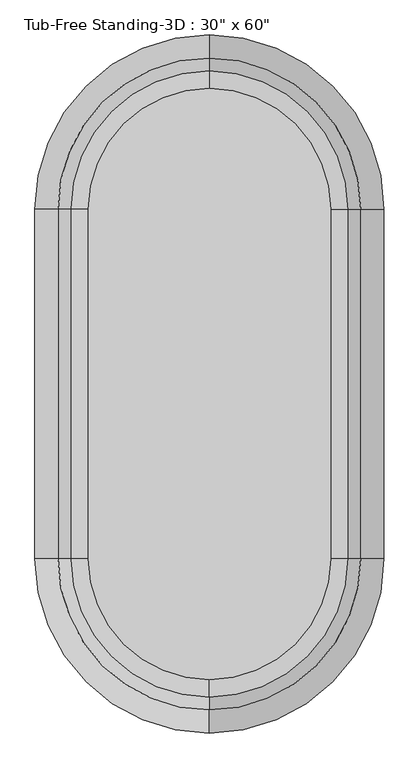
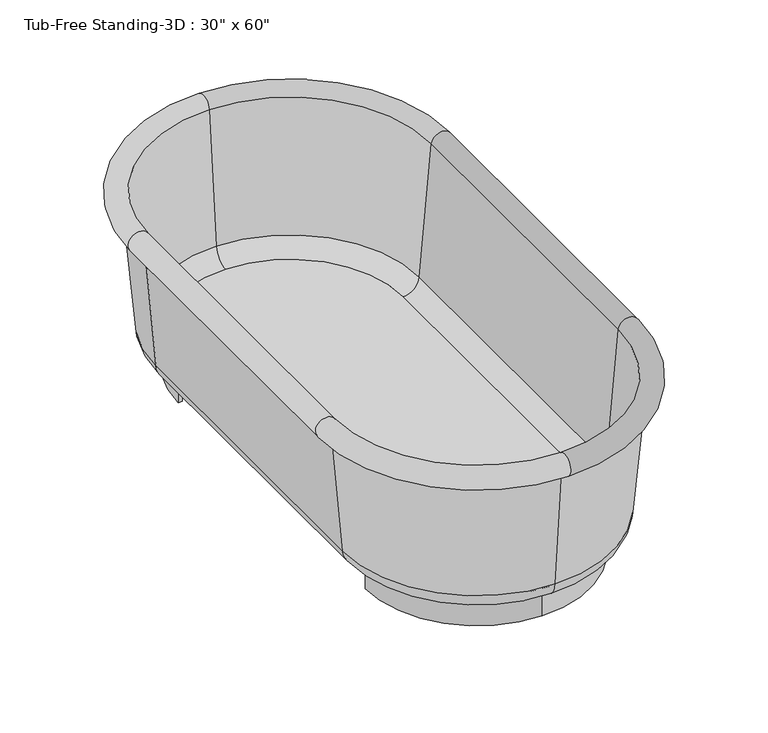
"""IFC4 building model written with IfcOpenShell, lengths in millimetres: flow terminal geometry."""

from ifc_helpers import new_model, si_unit, point, frame, frame_2d, origin, origin_with_axes, place, context, project, spatial, polyline, circle_curve, ellipse_curve, trimmed, segment, composite_curve, outline, extrude, source, transform, mapped, element, save
from ifc_brep_helpers import plane_surface, cylinder_surface, revolved_surface, advanced_brep


def flow_terminal_b374fae2(model_context):
    return source(origin(), model_context, "Body", "SolidModel", [
        extrude(outline(composite_curve([segment(trimmed(circle_curve(frame_2d((0.0, 381.0)), 254.0), [point((0.0, 635.0))], [point((-254.0, 381.0))], True, "CARTESIAN"), True, "CONTINUOUS"), segment(polyline([(-254.0, 381.0), (-264.2824236, 381.0)]), True, "CONTINUOUS"), segment(trimmed(circle_curve(frame_2d((0.0, 381.0)), 264.2824236), [point((-264.2824236, 381.0))], [point((0.0, 645.2824236))], False, "CARTESIAN"), True, "CONTINUOUS"), segment(trimmed(circle_curve(frame_2d((0.0, 381.0)), 264.2824236), [point((0.0, 645.2824236))], [point((264.2824236, 381.0))], False, "CARTESIAN"), True, "CONTINUOUS"), segment(polyline([(264.2824236, 381.0), (254.0, 381.0)]), True, "CONTINUOUS"), segment(trimmed(circle_curve(frame_2d((0.0, 381.0)), 254.0), [point((254.0, 381.0))], [point((0.0, 635.0))], True, "CARTESIAN"), True, "CONTINUOUS")], self_intersect=False)), origin_with_axes(), (0.0, 0.0, 1.0), 63.5),
        extrude(outline(composite_curve([segment(trimmed(circle_curve(frame_2d((0.0, -381.0)), 264.2824236), [point((0.0, -645.2824236))], [point((-264.2824236, -381.0))], False, "CARTESIAN"), True, "CONTINUOUS"), segment(polyline([(-264.2824236, -381.0), (-254.0, -381.0)]), True, "CONTINUOUS"), segment(trimmed(circle_curve(frame_2d((0.0, -381.0)), 254.0), [point((-254.0, -381.0))], [point((0.0, -635.0))], True, "CARTESIAN"), True, "CONTINUOUS"), segment(trimmed(circle_curve(frame_2d((0.0, -381.0)), 254.0), [point((0.0, -635.0))], [point((254.0, -381.0))], True, "CARTESIAN"), True, "CONTINUOUS"), segment(polyline([(254.0, -381.0), (264.2824236, -381.0)]), True, "CONTINUOUS"), segment(trimmed(circle_curve(frame_2d((0.0, -381.0)), 264.2824236), [point((264.2824236, -381.0))], [point((0.0, -645.2824236))], False, "CARTESIAN"), True, "CONTINUOUS")], self_intersect=False)), origin_with_axes(), (0.0, 0.0, 1.0), 63.5),
        extrude(outline(composite_curve([segment(polyline([(-264.2824236, -381.0), (-264.2824236, 381.0)]), True, "CONTINUOUS"), segment(trimmed(circle_curve(frame_2d((0.0, 381.0)), 264.2824236), [point((-264.2824236, 381.0))], [point((0.0, 645.2824236))], False, "CARTESIAN"), True, "CONTINUOUS"), segment(trimmed(circle_curve(frame_2d((0.0, 381.0)), 264.2824236), [point((0.0, 645.2824236))], [point((264.2824236, 381.0))], False, "CARTESIAN"), True, "CONTINUOUS"), segment(polyline([(264.2824236, 381.0), (264.2824236, -381.0)]), True, "CONTINUOUS"), segment(trimmed(circle_curve(frame_2d((0.0, -381.0)), 264.2824236), [point((264.2824236, -381.0))], [point((0.0, -645.2824236))], False, "CARTESIAN"), True, "CONTINUOUS"), segment(trimmed(circle_curve(frame_2d((0.0, -381.0)), 264.2824236), [point((0.0, -645.2824236))], [point((-264.2824236, -381.0))], False, "CARTESIAN"), True, "CONTINUOUS")], self_intersect=False)), frame((0.0, 0.0, 63.5), z_axis=(0.0, 0.0, 1.0), x_axis=(1.0, 0.0, 0.0)), (0.0, 0.0, 1.0), 15.08125),
        advanced_brep(
        [(0.0, -723.9, 406.4), (342.9, -381.0, 406.4), (355.6, -381.0, 406.4), (0.0, -736.6, 406.4), (0.0, -698.1045038, 111.5561295), (317.1045038, -381.0, 111.5561295), (0.0, -645.2824236, 63.1536107), (264.2824236, -381.0, 63.1536107), (0.0, -645.2824236, 78.0774627), (264.2824236, -381.0, 78.0774627), (0.0, -683.2374416, 112.8568289), (302.2374416, -381.0, 112.8568289), (0.0, -711.4561556, 435.3982063), (330.4561556, -381.0, 435.3982063), (-342.9, -381.0, 406.4), (-355.6, -381.0, 406.4), (-317.1045038, -381.0, 111.5561295), (-264.2824236, -381.0, 63.1536107), (-264.2824236, -381.0, 78.0774627), (-302.2374416, -381.0, 112.8568289), (-330.4561556, -381.0, 435.3982063), (-355.6, 381.0, 406.4), (-342.9, 381.0, 406.4), (-317.1045038, 381.0, 111.5561295), (-264.2824236, 381.0, 63.1536107), (-264.2824236, 381.0, 78.0774627), (-302.2374416, 381.0, 112.8568289), (-330.4561556, 381.0, 435.3982063), (0.0, 723.9, 406.4), (0.0, 736.6, 406.4), (0.0, 698.1045038, 111.5561295), (0.0, 645.2824236, 63.1536107), (0.0, 645.2824236, 78.0774627), (0.0, 683.2374416, 112.8568289), (0.0, 711.4561556, 435.3982063), (342.9, 381.0, 406.4), (355.6, 381.0, 406.4), (317.1045038, 381.0, 111.5561295), (264.2824236, 381.0, 63.1536107), (264.2824236, 381.0, 78.0774627), (302.2374416, 381.0, 112.8568289), (330.4561556, 381.0, 435.3982063)],
        [
            (0, 1, circle_curve(frame((0.0, -381.0, 406.4), z_axis=(0.0, 0.0, 1.0), x_axis=(1.0, 0.0, 0.0)), 342.9)),
            (1, 2),
            (2, 3, circle_curve(frame((0.0, -381.0, 406.4), z_axis=(0.0, 0.0, -1.0), x_axis=(1.0, 0.0, 0.0)), 355.6)),
            (3, 0),
            (4, 5, circle_curve(frame((0.0, -381.0, 111.5561295), z_axis=(0.0, 0.0, 1.0), x_axis=(1.0, 0.0, 0.0)), 317.1045038)),
            (5, 1),
            (0, 4),
            (6, 7, circle_curve(frame((0.0, -381.0, 63.1536107), z_axis=(0.0, 0.0, 1.0), x_axis=(1.0, 0.0, 0.0)), 264.2824236)),
            (7, 5, circle_curve(frame((264.2824236, -381.0, 116.1774627), z_axis=(0.0, -1.0, 0.0), x_axis=(1.0, 0.0, 0.0)), 53.023852)),
            (4, 6, circle_curve(frame((0.0, -645.2824236, 116.1774627), z_axis=(1.0, 0.0, 0.0), x_axis=(0.0, -1.0, 0.0)), 53.023852)),
            (8, 9, circle_curve(frame((0.0, -381.0, 78.0774627), z_axis=(0.0, 0.0, 1.0), x_axis=(1.0, 0.0, 0.0)), 264.2824236)),
            (9, 7),
            (6, 8),
            (10, 11, circle_curve(frame((0.0, -381.0, 112.8568289), z_axis=(0.0, 0.0, 1.0), x_axis=(1.0, 0.0, 0.0)), 302.2374416)),
            (11, 9, circle_curve(frame((264.2824236, -381.0, 116.1774627), z_axis=(0.0, 1.0, 0.0), x_axis=(1.0, 0.0, 0.0)), 38.1)),
            (8, 10, circle_curve(frame((0.0, -645.2824236, 116.1774627), z_axis=(-1.0, 0.0, 0.0), x_axis=(0.0, -1.0, 0.0)), 38.1)),
            (12, 13, circle_curve(frame((0.0, -381.0, 435.3982063), z_axis=(0.0, 0.0, 1.0), x_axis=(1.0, 0.0, 0.0)), 330.4561556)),
            (13, 11),
            (10, 12),
            (2, 13, circle_curve(frame((355.6, -381.0, 431.8), z_axis=(0.0, -1.0, 0.0), x_axis=(1.0, 0.0, 0.0)), 25.4)),
            (12, 3, circle_curve(frame((0.0, -736.6, 431.8), z_axis=(1.0, 0.0, 0.0), x_axis=(0.0, -1.0, 0.0)), 25.4)),
            (14, 0, circle_curve(frame((0.0, -381.0, 406.4), z_axis=(0.0, 0.0, 1.0), x_axis=(0.0, -1.0, 0.0)), 342.9)),
            (3, 15, circle_curve(frame((0.0, -381.0, 406.4), z_axis=(0.0, 0.0, -1.0), x_axis=(0.0, -1.0, 0.0)), 355.6)),
            (15, 14),
            (16, 4, circle_curve(frame((0.0, -381.0, 111.5561295), z_axis=(0.0, 0.0, 1.0), x_axis=(0.0, -1.0, 0.0)), 317.1045038)),
            (14, 16),
            (17, 6, circle_curve(frame((0.0, -381.0, 63.1536107), z_axis=(0.0, 0.0, 1.0), x_axis=(0.0, -1.0, 0.0)), 264.2824236)),
            (16, 17, circle_curve(frame((-264.2824236, -381.0, 116.1774627), z_axis=(0.0, -1.0, 0.0), x_axis=(-1.0, 0.0, 0.0)), 53.023852)),
            (18, 8, circle_curve(frame((0.0, -381.0, 78.0774627), z_axis=(0.0, 0.0, 1.0), x_axis=(0.0, -1.0, 0.0)), 264.2824236)),
            (17, 18),
            (19, 10, circle_curve(frame((0.0, -381.0, 112.8568289), z_axis=(0.0, 0.0, 1.0), x_axis=(0.0, -1.0, 0.0)), 302.2374416)),
            (18, 19, circle_curve(frame((-264.2824236, -381.0, 116.1774627), z_axis=(0.0, 1.0, 0.0), x_axis=(-1.0, 0.0, 0.0)), 38.1)),
            (20, 12, circle_curve(frame((0.0, -381.0, 435.3982063), z_axis=(0.0, 0.0, 1.0), x_axis=(0.0, -1.0, 0.0)), 330.4561556)),
            (19, 20),
            (20, 15, circle_curve(frame((-355.6, -381.0, 431.8), z_axis=(0.0, -1.0, 0.0), x_axis=(-1.0, 0.0, 0.0)), 25.4)),
            (15, 21),
            (21, 22),
            (22, 14),
            (22, 23),
            (23, 16),
            (23, 24, circle_curve(frame((-264.2824236, 381.0, 116.1774627), z_axis=(0.0, -1.0, 0.0), x_axis=(-1.0, 0.0, 0.0)), 53.023852)),
            (24, 17),
            (24, 25),
            (25, 18),
            (25, 26, circle_curve(frame((-264.2824236, 381.0, 116.1774627), z_axis=(0.0, 1.0, 0.0), x_axis=(-1.0, 0.0, 0.0)), 38.1)),
            (26, 19),
            (26, 27),
            (27, 20),
            (27, 21, circle_curve(frame((-355.6, 381.0, 431.8), z_axis=(0.0, -1.0, 0.0), x_axis=(-1.0, 0.0, 0.0)), 25.4)),
            (28, 22, circle_curve(frame((0.0, 381.0, 406.4), z_axis=(0.0, 0.0, 1.0), x_axis=(-1.0, 0.0, 0.0)), 342.9)),
            (21, 29, circle_curve(frame((0.0, 381.0, 406.4), z_axis=(0.0, 0.0, -1.0), x_axis=(-1.0, 0.0, 0.0)), 355.6)),
            (29, 28),
            (30, 23, circle_curve(frame((0.0, 381.0, 111.5561295), z_axis=(0.0, 0.0, 1.0), x_axis=(-1.0, 0.0, 0.0)), 317.1045038)),
            (28, 30),
            (31, 24, circle_curve(frame((0.0, 381.0, 63.1536107), z_axis=(0.0, 0.0, 1.0), x_axis=(-1.0, 0.0, 0.0)), 264.2824236)),
            (30, 31, circle_curve(frame((0.0, 645.2824236, 116.1774627), z_axis=(-1.0, 0.0, 0.0), x_axis=(0.0, 1.0, 0.0)), 53.023852)),
            (32, 25, circle_curve(frame((0.0, 381.0, 78.0774627), z_axis=(0.0, 0.0, 1.0), x_axis=(-1.0, 0.0, 0.0)), 264.2824236)),
            (31, 32),
            (33, 26, circle_curve(frame((0.0, 381.0, 112.8568289), z_axis=(0.0, 0.0, 1.0), x_axis=(-1.0, 0.0, 0.0)), 302.2374416)),
            (32, 33, circle_curve(frame((0.0, 645.2824236, 116.1774627), z_axis=(1.0, 0.0, 0.0), x_axis=(0.0, 1.0, 0.0)), 38.1)),
            (34, 27, circle_curve(frame((0.0, 381.0, 435.3982063), z_axis=(0.0, 0.0, 1.0), x_axis=(-1.0, 0.0, 0.0)), 330.4561556)),
            (33, 34),
            (34, 29, circle_curve(frame((0.0, 736.6, 431.8), z_axis=(-1.0, 0.0, 0.0), x_axis=(0.0, 1.0, 0.0)), 25.4)),
            (35, 28, circle_curve(frame((0.0, 381.0, 406.4), z_axis=(0.0, 0.0, 1.0), x_axis=(0.0, 1.0, 0.0)), 342.9)),
            (29, 36, circle_curve(frame((0.0, 381.0, 406.4), z_axis=(0.0, 0.0, -1.0), x_axis=(0.0, 1.0, 0.0)), 355.6)),
            (36, 35),
            (37, 30, circle_curve(frame((0.0, 381.0, 111.5561295), z_axis=(0.0, 0.0, 1.0), x_axis=(0.0, 1.0, 0.0)), 317.1045038)),
            (35, 37),
            (38, 31, circle_curve(frame((0.0, 381.0, 63.1536107), z_axis=(0.0, 0.0, 1.0), x_axis=(0.0, 1.0, 0.0)), 264.2824236)),
            (37, 38, circle_curve(frame((264.2824236, 381.0, 116.1774627), z_axis=(0.0, 1.0, 0.0), x_axis=(1.0, 0.0, 0.0)), 53.023852)),
            (39, 32, circle_curve(frame((0.0, 381.0, 78.0774627), z_axis=(0.0, 0.0, 1.0), x_axis=(0.0, 1.0, 0.0)), 264.2824236)),
            (38, 39),
            (40, 33, circle_curve(frame((0.0, 381.0, 112.8568289), z_axis=(0.0, 0.0, 1.0), x_axis=(0.0, 1.0, 0.0)), 302.2374416)),
            (39, 40, circle_curve(frame((264.2824236, 381.0, 116.1774627), z_axis=(0.0, -1.0, 0.0), x_axis=(1.0, 0.0, 0.0)), 38.1)),
            (41, 34, circle_curve(frame((0.0, 381.0, 435.3982063), z_axis=(0.0, 0.0, 1.0), x_axis=(0.0, 1.0, 0.0)), 330.4561556)),
            (40, 41),
            (41, 36, circle_curve(frame((355.6, 381.0, 431.8), z_axis=(0.0, 1.0, 0.0), x_axis=(1.0, 0.0, 0.0)), 25.4)),
            (36, 2),
            (1, 35),
            (5, 37),
            (7, 38),
            (9, 39),
            (11, 40),
            (13, 41),
        ],
        [
            plane_surface(frame((0.0, -381.0, 406.4), z_axis=(0.0, 0.0, -1.0), x_axis=(1.0, 0.0, 0.0))),
            revolved_surface(polyline([(342.9, -381.0, 406.4), (317.1045038, -381.0, 111.5561295)]), (0.0, -381.0, 431.8), (0.0, 0.0, -1.0)),
            revolved_surface(trimmed(ellipse_curve(frame((264.2824236, -381.0, 116.1774627), z_axis=(0.0, 1.0, 0.0), x_axis=(1.0, 0.0, 0.0)), 53.023852, 53.023852), [point((317.1045038, -381.0, 111.5561295))], [point((264.2824236, -381.0, 63.1536107))], True, "CARTESIAN"), (0.0, -381.0, 431.8), (0.0, 0.0, -1.0)),
            revolved_surface(polyline([(264.2824236, -381.0, 63.1536107), (264.2824236, -381.0, 78.07746270000001)]), (0.0, -381.0, 431.8), (0.0, 0.0, -1.0)),
            revolved_surface(trimmed(ellipse_curve(frame((264.2824236, -381.0, 116.1774627), z_axis=(0.0, -1.0, 0.0), x_axis=(1.0, 0.0, 0.0)), 38.1, 38.1), [point((264.2824236, -381.0, 78.0774627))], [point((302.2374416, -381.0, 112.8568289))], True, "CARTESIAN"), (0.0, -381.0, 431.8), (0.0, 0.0, -1.0)),
            revolved_surface(polyline([(302.2374416, -381.0, 112.8568289), (330.4561556, -381.0, 435.3982063)]), (0.0, -381.0, 431.8), (0.0, 0.0, -1.0)),
            revolved_surface(trimmed(ellipse_curve(frame((355.6, -381.0, 431.8), z_axis=(0.0, 1.0, 0.0), x_axis=(1.0, 0.0, 0.0)), 25.4, 25.4), [point((330.4561556, -381.0, 435.3982063))], [point((355.6, -381.0, 406.4))], True, "CARTESIAN"), (0.0, -381.0, 431.8), (0.0, 0.0, -1.0)),
            plane_surface(frame((0.0, -381.0, 406.4), z_axis=(0.0, 0.0, -1.0), x_axis=(0.0, -1.0, 0.0))),
            revolved_surface(polyline([(0.0, -723.9, 406.4), (0.0, -698.1045038, 111.5561295)]), (0.0, -381.0, 431.8), (0.0, 0.0, -1.0)),
            revolved_surface(trimmed(ellipse_curve(frame((0.0, -645.2824236, 116.1774627), z_axis=(1.0, 0.0, 0.0), x_axis=(0.0, -1.0, 0.0)), 53.023852, 53.023852), [point((0.0, -698.1045038, 111.5561295))], [point((0.0, -645.2824236, 63.1536107))], True, "CARTESIAN"), (0.0, -381.0, 431.8), (0.0, 0.0, -1.0)),
            revolved_surface(polyline([(0.0, -645.2824236, 63.1536107), (0.0, -645.2824236, 78.07746270000001)]), (0.0, -381.0, 431.8), (0.0, 0.0, -1.0)),
            revolved_surface(trimmed(ellipse_curve(frame((0.0, -645.2824236, 116.1774627), z_axis=(-1.0, 0.0, 0.0), x_axis=(0.0, -1.0, 0.0)), 38.1, 38.1), [point((0.0, -645.2824236, 78.0774627))], [point((0.0, -683.2374416, 112.8568289))], True, "CARTESIAN"), (0.0, -381.0, 431.8), (0.0, 0.0, -1.0)),
            revolved_surface(polyline([(0.0, -683.2374416, 112.8568289), (0.0, -711.4561556, 435.3982063)]), (0.0, -381.0, 431.8), (0.0, 0.0, -1.0)),
            revolved_surface(trimmed(ellipse_curve(frame((0.0, -736.6, 431.8), z_axis=(1.0, 0.0, 0.0), x_axis=(0.0, -1.0, 0.0)), 25.4, 25.4), [point((0.0, -711.4561556, 435.3982063))], [point((0.0, -736.6, 406.4))], True, "CARTESIAN"), (0.0, -381.0, 431.8), (0.0, 0.0, -1.0)),
            plane_surface(frame((-355.6, -381.0, 406.4), z_axis=(0.0, 0.0, -1.0), x_axis=(0.0, 1.0, 0.0))),
            plane_surface(frame((-342.9, -381.0, 406.4), z_axis=(-0.9961946980917455, 0.0, -0.08715574274765871), x_axis=(0.0, 1.0, 0.0))),
            cylinder_surface(frame((-264.2824236, -381.0, 116.1774627), z_axis=(0.0, -1.0, 0.0), x_axis=(-1.0, 0.0, 0.0)), 53.023852),
            plane_surface(frame((-264.2824236, -381.0, 63.1536107), z_axis=(1.0, 0.0, 0.0), x_axis=(0.0, 1.0, 0.0))),
            revolved_surface(polyline([(-302.38242360000004, 381.0, 116.1774627), (-302.38242360000004, -381.0, 116.1774627)]), (-264.2824236, -381.0, 116.1774627), (0.0, 1.0, 0.0)),
            plane_surface(frame((-302.2374416, -381.0, 112.8568289), z_axis=(0.9961946980917458, 0.0, 0.08715574274765651), x_axis=(0.0, 1.0, 0.0))),
            cylinder_surface(frame((-355.6, -381.0, 431.8), z_axis=(0.0, -1.0, 0.0), x_axis=(-1.0, 0.0, 0.0)), 25.4),
            plane_surface(frame((0.0, 381.0, 406.4), z_axis=(0.0, 0.0, -1.0), x_axis=(-1.0, 0.0, 0.0))),
            revolved_surface(polyline([(-342.9, 381.0, 406.4), (-317.1045038, 381.0, 111.5561295)]), (0.0, 381.0, 431.8), (0.0, 0.0, -1.0)),
            revolved_surface(trimmed(ellipse_curve(frame((-264.2824236, 381.0, 116.1774627), z_axis=(0.0, -1.0, 0.0), x_axis=(-1.0, 0.0, 0.0)), 53.023852, 53.023852), [point((-317.1045038, 381.0, 111.5561295))], [point((-264.2824236, 381.0, 63.1536107))], True, "CARTESIAN"), (0.0, 381.0, 431.8), (0.0, 0.0, -1.0)),
            revolved_surface(polyline([(-264.2824236, 381.0, 63.1536107), (-264.2824236, 381.0, 78.07746270000001)]), (0.0, 381.0, 431.8), (0.0, 0.0, -1.0)),
            revolved_surface(trimmed(ellipse_curve(frame((-264.2824236, 381.0, 116.1774627), z_axis=(0.0, 1.0, 0.0), x_axis=(-1.0, 0.0, 0.0)), 38.1, 38.1), [point((-264.2824236, 381.0, 78.0774627))], [point((-302.2374416, 381.0, 112.8568289))], True, "CARTESIAN"), (0.0, 381.0, 431.8), (0.0, 0.0, -1.0)),
            revolved_surface(polyline([(-302.2374416, 381.0, 112.8568289), (-330.4561556, 381.0, 435.3982063)]), (0.0, 381.0, 431.8), (0.0, 0.0, -1.0)),
            revolved_surface(trimmed(ellipse_curve(frame((-355.6, 381.0, 431.8), z_axis=(0.0, -1.0, 0.0), x_axis=(-1.0, 0.0, 0.0)), 25.4, 25.4), [point((-330.4561556, 381.0, 435.3982063))], [point((-355.6, 381.0, 406.4))], True, "CARTESIAN"), (0.0, 381.0, 431.8), (0.0, 0.0, -1.0)),
            plane_surface(frame((0.0, 381.0, 406.4), z_axis=(0.0, 0.0, -1.0), x_axis=(0.0, 1.0, 0.0))),
            revolved_surface(polyline([(0.0, 723.9, 406.4), (0.0, 698.1045038, 111.5561295)]), (0.0, 381.0, 431.8), (0.0, 0.0, -1.0)),
            revolved_surface(trimmed(ellipse_curve(frame((0.0, 645.2824236, 116.1774627), z_axis=(-1.0, 0.0, 0.0), x_axis=(0.0, 1.0, 0.0)), 53.023852, 53.023852), [point((0.0, 698.1045038, 111.5561295))], [point((0.0, 645.2824236, 63.1536107))], True, "CARTESIAN"), (0.0, 381.0, 431.8), (0.0, 0.0, -1.0)),
            revolved_surface(polyline([(0.0, 645.2824236, 63.1536107), (0.0, 645.2824236, 78.07746270000001)]), (0.0, 381.0, 431.8), (0.0, 0.0, -1.0)),
            revolved_surface(trimmed(ellipse_curve(frame((0.0, 645.2824236, 116.1774627), z_axis=(1.0, 0.0, 0.0), x_axis=(0.0, 1.0, 0.0)), 38.1, 38.1), [point((0.0, 645.2824236, 78.0774627))], [point((0.0, 683.2374416, 112.8568289))], True, "CARTESIAN"), (0.0, 381.0, 431.8), (0.0, 0.0, -1.0)),
            revolved_surface(polyline([(0.0, 683.2374416, 112.8568289), (0.0, 711.4561556, 435.3982063)]), (0.0, 381.0, 431.8), (0.0, 0.0, -1.0)),
            revolved_surface(trimmed(ellipse_curve(frame((0.0, 736.6, 431.8), z_axis=(-1.0, 0.0, 0.0), x_axis=(0.0, 1.0, 0.0)), 25.4, 25.4), [point((0.0, 711.4561556, 435.3982063))], [point((0.0, 736.6, 406.4))], True, "CARTESIAN"), (0.0, 381.0, 431.8), (0.0, 0.0, -1.0)),
            plane_surface(frame((355.6, 381.0, 406.4), z_axis=(0.0, 0.0, -1.0), x_axis=(0.0, -1.0, 0.0))),
            plane_surface(frame((342.9, 381.0, 406.4), z_axis=(0.9961946980917455, 0.0, -0.08715574274765871), x_axis=(0.0, -1.0, 0.0))),
            cylinder_surface(frame((264.2824236, 381.0, 116.1774627), z_axis=(0.0, 1.0, 0.0), x_axis=(1.0, 0.0, 0.0)), 53.023852),
            plane_surface(frame((264.2824236, 381.0, 63.1536107), z_axis=(-1.0, 0.0, 0.0), x_axis=(0.0, -1.0, 0.0))),
            revolved_surface(polyline([(302.38242360000004, -381.0, 116.1774627), (302.38242360000004, 381.0, 116.1774627)]), (264.2824236, 381.0, 116.1774627), (0.0, -1.0, 0.0)),
            plane_surface(frame((302.2374416, 381.0, 112.8568289), z_axis=(-0.9961946980917458, 0.0, 0.08715574274765651), x_axis=(0.0, -1.0, 0.0))),
            cylinder_surface(frame((355.6, 381.0, 431.8), z_axis=(0.0, 1.0, 0.0), x_axis=(1.0, 0.0, 0.0)), 25.4),
        ],
        [
            (0, [[1, 2, 3, 4]]),
            (1, [[5, 6, -1, 7]]),
            (2, [[8, 9, -5, 10]]),
            (3, [[11, 12, -8, 13]]),
            (4, [[14, 15, -11, 16]]),
            (5, [[17, 18, -14, 19]]),
            (6, [[-3, 20, -17, 21]]),
            (7, [[22, -4, 23, 24]]),
            (8, [[25, -7, -22, 26]]),
            (9, [[27, -10, -25, 28]]),
            (10, [[29, -13, -27, 30]]),
            (11, [[31, -16, -29, 32]]),
            (12, [[33, -19, -31, 34]]),
            (13, [[-23, -21, -33, 35]]),
            (14, [[-24, 36, 37, 38]]),
            (15, [[-26, -38, 39, 40]]),
            (16, [[-28, -40, 41, 42]]),
            (17, [[-30, -42, 43, 44]]),
            (18, [[-32, -44, 45, 46]]),
            (19, [[-34, -46, 47, 48]]),
            (20, [[-35, -48, 49, -36]]),
            (21, [[50, -37, 51, 52]]),
            (22, [[53, -39, -50, 54]]),
            (23, [[55, -41, -53, 56]]),
            (24, [[57, -43, -55, 58]]),
            (25, [[59, -45, -57, 60]]),
            (26, [[61, -47, -59, 62]]),
            (27, [[-51, -49, -61, 63]]),
            (28, [[64, -52, 65, 66]]),
            (29, [[67, -54, -64, 68]]),
            (30, [[69, -56, -67, 70]]),
            (31, [[71, -58, -69, 72]]),
            (32, [[73, -60, -71, 74]]),
            (33, [[75, -62, -73, 76]]),
            (34, [[-65, -63, -75, 77]]),
            (35, [[-66, 78, -2, 79]]),
            (36, [[-68, -79, -6, 80]]),
            (37, [[-70, -80, -9, 81]]),
            (38, [[-72, -81, -12, 82]]),
            (39, [[-74, -82, -15, 83]]),
            (40, [[-76, -83, -18, 84]]),
            (41, [[-77, -84, -20, -78]]),
        ],
    ),
    ])


if __name__ == "__main__":
    model = new_model("IFC4")
    model_context = context("Model", 3, world=origin())
    ifc_project = project(units=[si_unit("LENGTHUNIT", "METRE", prefix="MILLI")], contexts=[model_context])
    site = spatial("IfcSite", under=ifc_project)
    building = spatial("IfcBuilding", under=site)
    placement = place(None, origin())
    flow_terminal_shape = flow_terminal_b374fae2(model_context)
    element("IfcFlowTerminal", 1, ObjectType="Tub-Free Standing-3D : 30\" x 60\"", at=placement, inside=building, context=model_context, shape_type="MappedRepresentation", body=[
        mapped(flow_terminal_shape, transform((0.0, 0.0, 0.0), x_axis=(1.0, 0.0, 0.0), y_axis=(0.0, 1.0, 0.0), z_axis=(0.0, 0.0, 1.0))),
    ])
    save(model, "model.ifc")

# Revit data of these elements
# Type "Tub-Free Standing-3D : 30\" x 60\""
#   Assembly Code = "D2010110"
#   Height = 1' - 6"
#   Length = 5' - 0"
#   Width = 2' - 6"
#   Tub Material = Porcelain, Ivory
# Element 1 (IfcFlowTerminal, "Tub-Free Standing-3D : 30\" x 60\"")
#   Materials on its faces: "Porcelain, Ivory"
# Materials
#   "Porcelain, Ivory": class "Ceramic", colour RGB 247 247 239, transparency 0, Description = "Porcelain, ivory", Cost = 0
